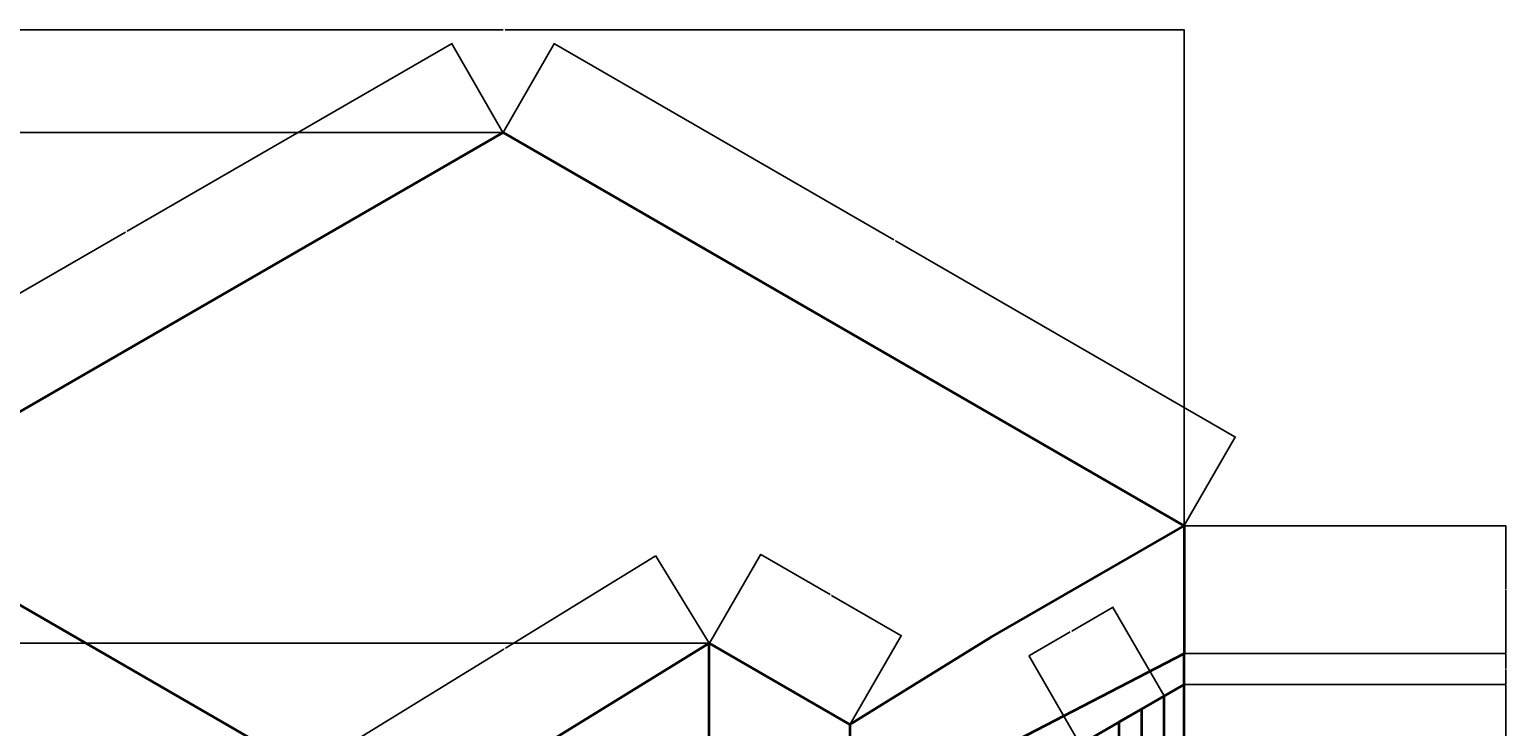
# Model space of a CAD drawing. Units: inches. Extents: x 61 to 939, y -128 to 676.
# Tile 3 of 3: x 355 to 939, y 400 to 676. Entities that reach past the tile are written whole.
import ezdxf

# ---------------------------------------------------------------- set-up
doc = ezdxf.new("R2010")
doc.units = ezdxf.units.IN
doc.header["$MEASUREMENT"] = 0
doc.layers.add('A-ANNO-DIMS', color=2, linetype='Continuous', lineweight=18)
doc.layers.add('A-ELEV', color=7, linetype='Continuous', lineweight=35)
doc.styles.get("Standard").update_dxf_attribs({"font": 'arial.ttf'})
doc.dimstyles.get("Standard").update_dxf_attribs({"dimtxt": 0.18, "dimasz": 0.18, "dimexe": 0.18, "dimexo": 0.0625, "dimgap": 0.09, "dimtad": 0, "dimtih": 1, "dimtoh": 1, "dimdec": 4, "dimzin": 0, "dimdsep": 46, "dimtxsty": 'Standard', "dimcen": 0.09, "dimadec": 0, "dimazin": 0, "dimtfac": 1, "dimtdec": 4, "dimtofl": 0, "dimtmove": 0, "dimatfit": 3, "dimfxl": 1, "dimtolj": 1, "dimtzin": 0, "dimarcsym": 0})

# ---------------------------------------------------------------- blocks, each defined once
blk = doc.blocks.new('*D1')
at = {"layer": 'A-ANNO-DIMS', "color": 0, "lineweight": -2, "transparency": 16777216}
for p, q in [((273.62, 289.95), (273.62, 675.84)), ((273.8, 675.66), (542.03, 675.66)), ((811.05, 675.66), (542.82, 675.66)), ((811.23, 479.78), (811.23, 675.84))]:
    blk.add_line(p, q, dxfattribs=at)
at = {"layer": 'A-ANNO-DIMS', "color": 0, "transparency": 16777216}
for points in [[(273.8, 675.69), (273.8, 675.63), (273.62, 675.66)], [(811.05, 675.69), (811.05, 675.63), (811.23, 675.66)]]:
    blk.add_solid(points, dxfattribs=at)
at = {"layer": 'Defpoints', "color": 0, "transparency": 16777216}
for p in [(811.23, 675.66), (811.23, 479.72), (273.62, 289.89)]:
    blk.add_point(p, dxfattribs=at)
at = {"layer": 'A-ANNO-DIMS', "color": 0, "transparency": 16777216, "insert": (542.42, 675.66), "char_height": 0.18, "attachment_point": 5}
blk.add_mtext('\\A1;537.6', dxfattribs=at)
blk = doc.blocks.new('*D2')
at = {"layer": 'A-ANNO-DIMS', "color": 0, "lineweight": -2, "transparency": 16777216}
for p, q in [((541.93, 635.16), (60.74, 635.16)), ((60.92, 634.98), (60.92, 273.9)), ((60.92, -87.54), (60.92, 273.54)), ((524.15, -87.72), (60.74, -87.72))]:
    blk.add_line(p, q, dxfattribs=at)
at = {"layer": 'A-ANNO-DIMS', "color": 0, "transparency": 16777216}
for points in [[(60.89, 634.98), (60.95, 634.98), (60.92, 635.16)], [(60.89, -87.54), (60.95, -87.54), (60.92, -87.72)]]:
    blk.add_solid(points, dxfattribs=at)
at = {"layer": 'Defpoints', "color": 0, "transparency": 16777216}
for p in [(60.92, 635.16), (542, 635.16), (524.21, -87.72)]:
    blk.add_point(p, dxfattribs=at)
at = {"layer": 'A-ANNO-DIMS', "color": 0, "transparency": 16777216, "insert": (60.92, 273.72), "char_height": 0.18, "attachment_point": 5}
blk.add_mtext('\\A1;722.9', dxfattribs=at)
blk = doc.blocks.new('*D6')
at = {"layer": 'A-ANNO-DIMS', "color": 0, "lineweight": -2, "transparency": 16777216}
for p, q in [((811.29, 416.97), (938.57, 416.97)), ((938.39, 416.79), (938.39, 375.11)), ((938.39, 333.08), (938.39, 374.75)), ((811.29, 332.9), (938.57, 332.9))]:
    blk.add_line(p, q, dxfattribs=at)
at = {"layer": 'A-ANNO-DIMS', "color": 0, "transparency": 16777216}
for points in [[(938.36, 416.79), (938.42, 416.79), (938.39, 416.97)], [(938.36, 333.08), (938.42, 333.08), (938.39, 332.9)]]:
    blk.add_solid(points, dxfattribs=at)
at = {"layer": 'Defpoints', "color": 0, "transparency": 16777216}
for p in [(811.23, 416.97), (938.39, 416.97), (811.23, 332.9)]:
    blk.add_point(p, dxfattribs=at)
at = {"layer": 'A-ANNO-DIMS', "color": 0, "transparency": 16777216, "insert": (938.39, 374.93), "char_height": 0.18, "attachment_point": 5}
blk.add_mtext('\\A1;84.07', dxfattribs=at)
blk = doc.blocks.new('*D7')
at = {"layer": 'A-ANNO-DIMS', "color": 0, "lineweight": -2, "transparency": 16777216}
for p, q in [((811.29, 429.21), (938.57, 429.21)), ((938.39, 429.03), (938.39, 423.27)), ((938.39, 417.15), (938.39, 422.91)), ((811.29, 416.97), (938.57, 416.97))]:
    blk.add_line(p, q, dxfattribs=at)
at = {"layer": 'A-ANNO-DIMS', "color": 0, "transparency": 16777216}
for points in [[(938.36, 429.03), (938.42, 429.03), (938.39, 429.21)], [(938.36, 417.15), (938.42, 417.15), (938.39, 416.97)]]:
    blk.add_solid(points, dxfattribs=at)
at = {"layer": 'Defpoints', "color": 0, "transparency": 16777216}
for p in [(811.23, 429.21), (938.39, 429.21), (811.23, 416.97)]:
    blk.add_point(p, dxfattribs=at)
at = {"layer": 'A-ANNO-DIMS', "color": 0, "transparency": 16777216, "insert": (938.39, 423.09), "char_height": 0.18, "attachment_point": 5}
blk.add_mtext('\\A1;12.24', dxfattribs=at)
blk = doc.blocks.new('*D8')
at = {"layer": 'A-ANNO-DIMS', "color": 0, "lineweight": -2, "transparency": 16777216}
for p, q in [((811.29, 479.72), (938.57, 479.72)), ((938.39, 479.54), (938.39, 454.64)), ((938.39, 429.39), (938.39, 454.28)), ((811.29, 429.21), (938.57, 429.21))]:
    blk.add_line(p, q, dxfattribs=at)
at = {"layer": 'A-ANNO-DIMS', "color": 0, "transparency": 16777216}
for points in [[(938.36, 479.54), (938.42, 479.54), (938.39, 479.72)], [(938.36, 429.39), (938.42, 429.39), (938.39, 429.21)]]:
    blk.add_solid(points, dxfattribs=at)
at = {"layer": 'Defpoints', "color": 0, "transparency": 16777216}
for p in [(811.23, 479.72), (938.39, 479.72), (811.23, 429.21)]:
    blk.add_point(p, dxfattribs=at)
at = {"layer": 'A-ANNO-DIMS', "color": 0, "transparency": 16777216, "insert": (938.39, 454.46), "char_height": 0.18, "attachment_point": 5}
blk.add_mtext('\\A1;50.51', dxfattribs=at)
blk = doc.blocks.new('*D28')
at = {"layer": 'A-ANNO-DIMS', "color": 0, "lineweight": -2, "transparency": 16777216}
for p, q in [((521.59, 670.14), (393.44, 596.16)), ((541.96, 635.21), (521.66, 670.39)), ((264.66, 521.8), (392.81, 595.79)), ((284.72, 486.69), (264.41, 521.87))]:
    blk.add_line(p, q, dxfattribs=at)
at = {"layer": 'A-ANNO-DIMS', "color": 0, "transparency": 16777216}
for points in [[(521.57, 670.17), (521.6, 670.12), (521.75, 670.23)], [(264.64, 521.83), (264.67, 521.78), (264.5, 521.71)]]:
    blk.add_solid(points, dxfattribs=at)
at = {"layer": 'Defpoints', "color": 0, "transparency": 16777216}
for p in [(521.75, 670.23), (542, 635.16), (284.75, 486.64)]:
    blk.add_point(p, dxfattribs=at)
at = {"layer": 'A-ANNO-DIMS', "color": 0, "transparency": 16777216, "insert": (393.12, 595.97), "char_height": 0.18, "attachment_point": 5}
blk.add_mtext('\\A1;297.04', dxfattribs=at)
blk = doc.blocks.new('*D29')
at = {"layer": 'A-ANNO-DIMS', "color": 0, "lineweight": -2, "transparency": 16777216}
for p, q in [((542.03, 635.21), (562.34, 670.39)), ((562.4, 670.14), (696.55, 592.69)), ((831.32, 514.88), (697.18, 592.33)), ((811.26, 479.77), (831.57, 514.95))]:
    blk.add_line(p, q, dxfattribs=at)
at = {"layer": 'A-ANNO-DIMS', "color": 0, "transparency": 16777216}
for points in [[(562.42, 670.17), (562.39, 670.12), (562.25, 670.23)], [(831.34, 514.91), (831.31, 514.86), (831.48, 514.79)]]:
    blk.add_solid(points, dxfattribs=at)
at = {"layer": 'Defpoints', "color": 0, "transparency": 16777216}
for p in [(542, 635.16), (831.48, 514.79), (811.23, 479.72)]:
    blk.add_point(p, dxfattribs=at)
at = {"layer": 'A-ANNO-DIMS', "color": 0, "transparency": 16777216, "insert": (696.86, 592.51), "char_height": 0.18, "attachment_point": 5}
blk.add_mtext('\\A1;310.89', dxfattribs=at)
blk = doc.blocks.new('*D30')
at = {"layer": 'A-ANNO-DIMS', "color": 0, "lineweight": -2, "transparency": 16777216}
for p, q in [((602.19, 467.71), (542.96, 431.31)), ((623.52, 433.36), (602.25, 467.96)), ((483.13, 394.55), (542.37, 430.95)), ((504.15, 360), (482.88, 394.61))]:
    blk.add_line(p, q, dxfattribs=at)
at = {"layer": 'A-ANNO-DIMS', "color": 0, "transparency": 16777216}
for points in [[(602.17, 467.74), (602.21, 467.69), (602.34, 467.81)], [(483.12, 394.58), (483.15, 394.52), (482.98, 394.46)]]:
    blk.add_solid(points, dxfattribs=at)
at = {"layer": 'Defpoints', "color": 0, "transparency": 16777216}
for p in [(602.34, 467.81), (623.55, 433.3), (504.18, 359.95)]:
    blk.add_point(p, dxfattribs=at)
at = {"layer": 'A-ANNO-DIMS', "color": 0, "transparency": 16777216, "insert": (542.66, 431.13), "char_height": 0.18, "attachment_point": 5}
blk.add_mtext('\\A1;140.10', dxfattribs=at)
blk = doc.blocks.new('*D31')
at = {"layer": 'A-ANNO-DIMS', "color": 0, "lineweight": -2, "transparency": 16777216}
for p, q in [((623.58, 433.36), (643.89, 468.53)), ((643.95, 468.29), (671.28, 452.51)), ((699.24, 436.37), (671.91, 452.14)), ((679.18, 401.26), (699.49, 436.43))]:
    blk.add_line(p, q, dxfattribs=at)
at = {"layer": 'A-ANNO-DIMS', "color": 0, "transparency": 16777216}
for points in [[(643.97, 468.31), (643.94, 468.26), (643.8, 468.38)], [(699.26, 436.39), (699.23, 436.34), (699.4, 436.28)]]:
    blk.add_solid(points, dxfattribs=at)
at = {"layer": 'Defpoints', "color": 0, "transparency": 16777216}
for p in [(623.55, 433.3), (699.4, 436.28), (679.15, 401.2)]:
    blk.add_point(p, dxfattribs=at)
at = {"layer": 'A-ANNO-DIMS', "color": 0, "transparency": 16777216, "insert": (671.6, 452.33), "char_height": 0.18, "attachment_point": 5}
blk.add_mtext('\\A1;64.20', dxfattribs=at)
blk = doc.blocks.new('*D32')
at = {"layer": 'A-ANNO-DIMS', "color": 0, "lineweight": -2, "transparency": 16777216}
for p, q in [((623.49, 433.3), (60.74, 433.3)), ((60.92, 433.12), (60.92, 411.64)), ((60.92, 389.79), (60.92, 411.27)), ((623.49, 389.61), (60.74, 389.61))]:
    blk.add_line(p, q, dxfattribs=at)
at = {"layer": 'A-ANNO-DIMS', "color": 0, "transparency": 16777216}
for points in [[(60.89, 433.12), (60.95, 433.12), (60.92, 433.3)], [(60.89, 389.79), (60.95, 389.79), (60.92, 389.61)]]:
    blk.add_solid(points, dxfattribs=at)
at = {"layer": 'Defpoints', "color": 0, "transparency": 16777216}
for p in [(623.55, 433.3), (60.92, 389.61), (623.55, 389.61)]:
    blk.add_point(p, dxfattribs=at)
at = {"layer": 'A-ANNO-DIMS', "color": 0, "transparency": 16777216, "insert": (60.92, 411.46), "char_height": 0.18, "attachment_point": 5}
blk.add_mtext('\\A1;43.695', dxfattribs=at)
blk = doc.blocks.new('*D38')
at = {"layer": 'A-ANNO-DIMS', "color": 0, "lineweight": -2, "transparency": 16777216}
for p, q in [((782.94, 447.4), (766.82, 438.09)), ((803.31, 412.47), (783, 447.65)), ((750.07, 428.42), (766.19, 437.73)), ((770.13, 393.31), (749.82, 428.49))]:
    blk.add_line(p, q, dxfattribs=at)
at = {"layer": 'A-ANNO-DIMS', "color": 0, "transparency": 16777216}
for points in [[(782.92, 447.43), (782.95, 447.37), (783.09, 447.49)], [(750.06, 428.45), (750.09, 428.4), (749.91, 428.33)]]:
    blk.add_solid(points, dxfattribs=at)
at = {"layer": 'Defpoints', "color": 0, "transparency": 16777216}
for p in [(783.09, 447.49), (803.34, 412.42), (770.16, 393.26)]:
    blk.add_point(p, dxfattribs=at)
at = {"layer": 'A-ANNO-DIMS', "color": 0, "transparency": 16777216, "insert": (766.5, 437.91), "char_height": 0.18, "attachment_point": 5}
blk.add_mtext('\\A1;38.31', dxfattribs=at)

msp = doc.modelspace()

# ---------------------------------------------------------------- linework, layer by layer
at = {"layer": 'A-ELEV'}
for p, q in [((284.7507, 486.6398), (541.9952, 635.1599)), ((811.2295, 479.7174), (541.9952, 635.1599)), ((734.7429, 435.5578), (811.2295, 479.7174)), ((811.2295, 479.7174), (811.2295, 429.2088)), ((504.1826, 359.9507), (325.5789, 463.0676)), ((623.5481, 433.303), (504.1826, 359.9507)), ((623.5481, 389.6079), (623.5481, 433.303)), ((623.5481, 433.303), (679.1474, 401.2027)), ((734.7429, 435.5578), (679.1474, 401.2027)), ((734.7429, 389.6058), (811.2295, 429.2088)), ((811.2295, 113.7993), (811.2295, 429.2088)), ((752.0802, 382.8189), (811.2295, 416.9688)), ((803.3445, 328.6095), (803.3445, 412.4164)), ((785.5849, 402.1629), (794.4408, 407.2759)), ((794.4408, 407.2759), (794.4408, 323.7678)), ((679.1474, 401.2027), (679.1474, 357.5076)), ((785.5849, 318.9521), (785.5849, 402.1629))]:
    msp.add_line(p, q, dxfattribs=at)

# ---------------------------------------------------------------- dimensions: what is measured, and where the dimension line sits
at = {"layer": 'A-ANNO-DIMS'}
dim = msp.add_linear_dim(base=(811.2295, 675.6599), p1=(273.6173, 289.886), p2=(811.2295, 479.7174), dimstyle='Standard', override={"dimdec": 1, "dimlfac": 1, "dimrnd": 0, "dimzin": 0, "dimdsep": 46, "dimlunit": 2}, dxfattribs=at)
dim.commit()
dim.dimension.update_dxf_attribs({"geometry": '*D1', "text_midpoint": (542.4234, 675.6599)})
for base, p1, p2, angle, override, picture, middle in [((521.7452, 670.2339), (284.7507, 486.6398), (541.9952, 635.1599), 30, {"dimdec": 2, "dimlfac": 1, "dimrnd": 0, "dimzin": 0, "dimdsep": 46, "dimlunit": 2}, '*D28', (393.1229, 595.9738)), ((831.47948, 514.79139), (541.99515, 635.15988), (811.22948, 479.71736), 330, {"dimdec": 2, "dimlfac": 1, "dimrnd": 0, "dimzin": 0, "dimdsep": 46, "dimlunit": 2}, '*D29', (696.86232, 592.51265)), ((60.9156, 635.1599), (524.212, -87.7241), (541.9952, 635.1599), 90, {"dimdec": 1, "dimlfac": 1, "dimrnd": 0, "dimzin": 0, "dimdsep": 46, "dimlunit": 2}, '*D2', (60.9156, 273.7179)), ((938.3863, 479.7174), (811.2295, 429.2088), (811.2295, 479.7174), 90, {"dimdec": 2, "dimlfac": 1, "dimrnd": 0, "dimzin": 0, "dimdsep": 46, "dimlunit": 2}, '*D8', (938.3863, 454.4631)), ((602.3439, 467.8085), (504.1826, 359.9507), (623.5481, 433.303), 31.5714469, {"dimdec": 2, "dimlfac": 1, "dimrnd": 0, "dimzin": 0, "dimdsep": 46, "dimlunit": 2}, '*D30', (542.6611, 431.1324)), ((699.3974, 436.2767), (623.5481, 433.303), (679.1474, 401.2027), 330, {"dimdec": 2, "dimlfac": 1, "dimrnd": 0, "dimzin": 0, "dimdsep": 46, "dimlunit": 2}, '*D31', (671.5978, 452.3269)), ((783.0945, 447.4905), (770.1647, 393.2601), (803.3445, 412.4164), 30, {"dimdec": 2, "dimlfac": 1, "dimrnd": 0, "dimzin": 0, "dimdsep": 46, "dimlunit": 2}, '*D38', (766.5046, 437.9123)), ((60.9156, 389.6079), (623.5481, 433.303), (623.5481, 389.6079), 90, {"dimdec": 3, "dimlfac": 1, "dimrnd": 0, "dimzin": 0, "dimdsep": 46, "dimlunit": 2}, '*D32', (60.9156, 411.4554)), ((938.3863, 429.2088), (811.2295, 416.9688), (811.2295, 429.2088), 90, {"dimdec": 2, "dimlfac": 1, "dimrnd": 0, "dimzin": 0, "dimdsep": 46, "dimlunit": 2}, '*D7', (938.3863, 423.0888)), ((938.3863, 416.9688), (811.2295, 332.8972), (811.2295, 416.9688), 90, {"dimdec": 2, "dimlfac": 1, "dimrnd": 0, "dimzin": 0, "dimdsep": 46, "dimlunit": 2}, '*D6', (938.3863, 374.933))]:
    dim = msp.add_linear_dim(base=base, p1=p1, p2=p2, angle=angle, dimstyle='Standard', override=override, dxfattribs=at)
    dim.commit()
    dim.dimension.update_dxf_attribs({"geometry": picture, "text_midpoint": middle})

doc.saveas('drawing.dxf')
